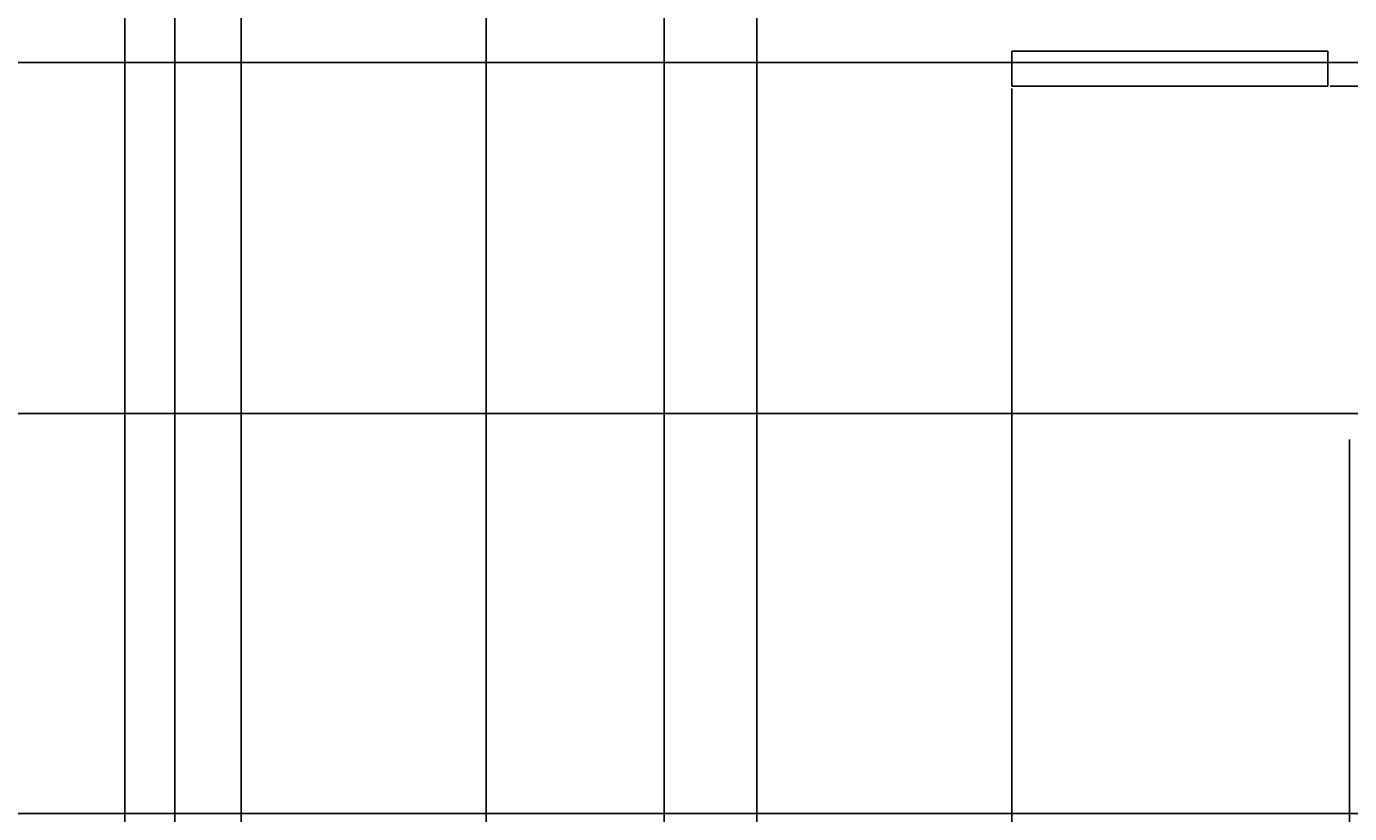
# Model space of a CAD drawing. Units: inches. Extents: x 2812 to 3051, y 1398 to 1659.
# Tile 30 of 65: x 2966 to 3004, y 1416 to 1438. Entities that reach past the tile are written whole.
import ezdxf

# ---------------------------------------------------------------- set-up
doc = ezdxf.new("R2010")
doc.units = ezdxf.units.IN
doc.layers.add('A-ANNO-DIMS', color=2, linetype='Continuous', lineweight=18)
doc.layers.add('S-STEP', color=3, linetype='Continuous', lineweight=25)
doc.styles.get("Standard").update_dxf_attribs({"font": 'arial.ttf'})
doc.dimstyles.get("Standard").update_dxf_attribs({"dimtxt": 0.18, "dimasz": 0.18, "dimexe": 0.18, "dimexo": 0.0625, "dimgap": 0.09, "dimtad": 0, "dimtih": 1, "dimtoh": 1, "dimdec": 4, "dimzin": 0, "dimdsep": 46, "dimtxsty": 'Standard', "dimcen": 0.09, "dimadec": 0, "dimazin": 0, "dimtfac": 1, "dimtdec": 4, "dimtofl": 0, "dimtmove": 0, "dimatfit": 3, "dimfxl": 1, "dimtolj": 1, "dimtzin": 0, "dimarcsym": 0})

# ---------------------------------------------------------------- blocks, each defined once
blk = doc.blocks.new('STEP-IRON-2')
for p, q in [((9, 1), (0, 1)), ((0, 1), (0, 0)), ((9, 0), (9, 1)), ((0, 0), (3.641, 0)), ((0, 0), (9, 0)), ((0, 0), (5.792, 0))]:
    blk.add_line(p, q)
blk = doc.blocks.new('*D31')
at = {"layer": 'A-ANNO-DIMS', "color": 0, "lineweight": -2, "transparency": 16777216}
for p, q in [((2972.272, 1594.192), (2972.272, 1397.505)), ((2961.385, 1559.757), (2961.385, 1397.505)), ((2961.565, 1397.685), (2966.373, 1397.685)), ((2972.092, 1397.685), (2967.283, 1397.685))]:
    blk.add_line(p, q, dxfattribs=at)
at = {"layer": 'A-ANNO-DIMS', "color": 0, "transparency": 16777216}
for points in [[(2961.565, 1397.715), (2961.565, 1397.655), (2961.385, 1397.685)], [(2972.092, 1397.715), (2972.092, 1397.655), (2972.272, 1397.685)]]:
    blk.add_solid(points, dxfattribs=at)
at = {"layer": 'Defpoints', "color": 0, "transparency": 16777216}
for p in [(2972.272, 1594.254), (2961.385, 1559.82), (2972.272, 1397.685)]:
    blk.add_point(p, dxfattribs=at)
at = {"layer": 'A-ANNO-DIMS', "color": 0, "transparency": 16777216, "insert": (2966.828, 1397.685), "char_height": 0.18, "attachment_point": 5}
blk.add_mtext('\\A1;10.887', dxfattribs=at)
blk = doc.blocks.new('*D32')
at = {"layer": 'A-ANNO-DIMS', "color": 0, "lineweight": -2, "transparency": 16777216}
for p, q in [((2984.316, 1598.757), (2984.316, 1397.505)), ((2972.272, 1594.192), (2972.272, 1397.505)), ((2972.452, 1397.685), (2977.839, 1397.685)), ((2984.136, 1397.685), (2978.748, 1397.685))]:
    blk.add_line(p, q, dxfattribs=at)
at = {"layer": 'A-ANNO-DIMS', "color": 0, "transparency": 16777216}
for points in [[(2972.452, 1397.715), (2972.452, 1397.655), (2972.272, 1397.685)], [(2984.136, 1397.715), (2984.136, 1397.655), (2984.316, 1397.685)]]:
    blk.add_solid(points, dxfattribs=at)
at = {"layer": 'Defpoints', "color": 0, "transparency": 16777216}
for p in [(2984.316, 1598.82), (2972.272, 1594.254), (2984.316, 1397.685)]:
    blk.add_point(p, dxfattribs=at)
at = {"layer": 'A-ANNO-DIMS', "color": 0, "transparency": 16777216, "insert": (2978.294, 1397.685), "char_height": 0.18, "attachment_point": 5}
blk.add_mtext('\\A1;12.044', dxfattribs=at)
blk = doc.blocks.new('*D46')
at = {"layer": 'A-ANNO-DIMS', "color": 0, "lineweight": -2, "transparency": 16777216}
for p, q in [((2941.385, 1487.973), (2941.385, 1397.505)), ((2970.385, 1487.973), (2970.385, 1397.505)), ((2941.565, 1397.685), (2955.664, 1397.685)), ((2970.205, 1397.685), (2956.106, 1397.685))]:
    blk.add_line(p, q, dxfattribs=at)
at = {"layer": 'A-ANNO-DIMS', "color": 0, "transparency": 16777216}
for points in [[(2941.565, 1397.715), (2941.565, 1397.655), (2941.385, 1397.685)], [(2970.205, 1397.715), (2970.205, 1397.655), (2970.385, 1397.685)]]:
    blk.add_solid(points, dxfattribs=at)
at = {"layer": 'Defpoints', "color": 0, "transparency": 16777216}
for p in [(2941.385, 1488.035), (2970.385, 1488.035), (2970.385, 1397.685)]:
    blk.add_point(p, dxfattribs=at)
at = {"layer": 'A-ANNO-DIMS', "color": 0, "transparency": 16777216, "insert": (2955.885, 1397.685), "char_height": 0.18, "attachment_point": 5}
blk.add_mtext('\\A1;29', dxfattribs=at)
blk = doc.blocks.new('*D47')
at = {"layer": 'A-ANNO-DIMS', "color": 0, "lineweight": -2, "transparency": 16777216}
for p, q in [((2970.385, 1487.973), (2970.385, 1397.505)), ((3006.385, 1487.973), (3006.385, 1397.505)), ((2970.565, 1397.685), (2988.166, 1397.685)), ((3006.205, 1397.685), (2988.604, 1397.685))]:
    blk.add_line(p, q, dxfattribs=at)
at = {"layer": 'A-ANNO-DIMS', "color": 0, "transparency": 16777216}
for points in [[(2970.565, 1397.715), (2970.565, 1397.655), (2970.385, 1397.685)], [(3006.205, 1397.715), (3006.205, 1397.655), (3006.385, 1397.685)]]:
    blk.add_solid(points, dxfattribs=at)
at = {"layer": 'Defpoints', "color": 0, "transparency": 16777216}
for p in [(2970.385, 1488.035), (3006.385, 1488.035), (3006.385, 1397.685)]:
    blk.add_point(p, dxfattribs=at)
at = {"layer": 'A-ANNO-DIMS', "color": 0, "transparency": 16777216, "insert": (2988.385, 1397.685), "char_height": 0.18, "attachment_point": 5}
blk.add_mtext('\\A1;36', dxfattribs=at)
blk = doc.blocks.new('*D64')
at = {"layer": 'A-ANNO-DIMS', "color": 0, "lineweight": -2, "transparency": 16777216}
for p, q in [((2929.438, 1427.426), (3051.178, 1427.426)), ((3050.998, 1427.246), (3050.998, 1421.913)), ((3050.998, 1416.215), (3050.998, 1421.549)), ((2952.447, 1416.035), (3051.178, 1416.035))]:
    blk.add_line(p, q, dxfattribs=at)
at = {"layer": 'A-ANNO-DIMS', "color": 0, "transparency": 16777216}
for points in [[(3050.968, 1427.246), (3051.028, 1427.246), (3050.998, 1427.426)], [(3050.968, 1416.215), (3051.028, 1416.215), (3050.998, 1416.035)]]:
    blk.add_solid(points, dxfattribs=at)
at = {"layer": 'Defpoints', "color": 0, "transparency": 16777216}
for p in [(2929.375, 1427.426), (3050.998, 1427.426), (2952.385, 1416.035)]:
    blk.add_point(p, dxfattribs=at)
at = {"layer": 'A-ANNO-DIMS', "color": 0, "transparency": 16777216, "insert": (3050.998, 1421.731), "char_height": 0.18, "attachment_point": 5}
blk.add_mtext('\\A1;11.39', dxfattribs=at)
blk = doc.blocks.new('*D65')
at = {"layer": 'A-ANNO-DIMS', "color": 0, "lineweight": -2, "transparency": 16777216}
for p, q in [((2920.62, 1437.426), (3051.178, 1437.426)), ((3050.998, 1437.246), (3050.998, 1432.608)), ((3050.998, 1427.606), (3050.998, 1432.245)), ((2929.438, 1427.426), (3051.178, 1427.426))]:
    blk.add_line(p, q, dxfattribs=at)
at = {"layer": 'A-ANNO-DIMS', "color": 0, "transparency": 16777216}
for points in [[(3050.968, 1437.246), (3051.028, 1437.246), (3050.998, 1437.426)], [(3050.968, 1427.606), (3051.028, 1427.606), (3050.998, 1427.426)]]:
    blk.add_solid(points, dxfattribs=at)
at = {"layer": 'Defpoints', "color": 0, "transparency": 16777216}
for p in [(2920.558, 1437.426), (3050.998, 1437.426), (2929.375, 1427.426)]:
    blk.add_point(p, dxfattribs=at)
at = {"layer": 'A-ANNO-DIMS', "color": 0, "transparency": 16777216, "insert": (3050.998, 1432.426), "char_height": 0.18, "attachment_point": 5}
blk.add_mtext('\\A1;10', dxfattribs=at)
blk = doc.blocks.new('*D66')
at = {"layer": 'A-ANNO-DIMS', "color": 0, "lineweight": -2, "transparency": 16777216}
for p, q in [((2914.018, 1447.426), (3051.178, 1447.426)), ((3050.998, 1447.246), (3050.998, 1442.608)), ((3050.998, 1437.606), (3050.998, 1442.245)), ((2920.62, 1437.426), (3051.178, 1437.426))]:
    blk.add_line(p, q, dxfattribs=at)
at = {"layer": 'A-ANNO-DIMS', "color": 0, "transparency": 16777216}
for points in [[(3050.968, 1447.246), (3051.028, 1447.246), (3050.998, 1447.426)], [(3050.968, 1437.606), (3051.028, 1437.606), (3050.998, 1437.426)]]:
    blk.add_solid(points, dxfattribs=at)
at = {"layer": 'Defpoints', "color": 0, "transparency": 16777216}
for p in [(2913.955, 1447.426), (3050.998, 1447.426), (2920.558, 1437.426)]:
    blk.add_point(p, dxfattribs=at)
at = {"layer": 'A-ANNO-DIMS', "color": 0, "transparency": 16777216, "insert": (3050.998, 1442.426), "char_height": 0.18, "attachment_point": 5}
blk.add_mtext('\\A1;10', dxfattribs=at)
blk = doc.blocks.new('*D71')
at = {"layer": 'A-ANNO-DIMS', "color": 0, "lineweight": -2, "transparency": 16777216}
for p, q in [((2968.956, 1466.685), (2968.956, 1397.505)), ((2979.248, 1456.685), (2979.248, 1397.505)), ((2969.136, 1397.685), (2973.648, 1397.685)), ((2979.068, 1397.685), (2974.556, 1397.685))]:
    blk.add_line(p, q, dxfattribs=at)
at = {"layer": 'A-ANNO-DIMS', "color": 0, "transparency": 16777216}
for points in [[(2969.136, 1397.715), (2969.136, 1397.655), (2968.956, 1397.685)], [(2979.068, 1397.715), (2979.068, 1397.655), (2979.248, 1397.685)]]:
    blk.add_solid(points, dxfattribs=at)
at = {"layer": 'Defpoints', "color": 0, "transparency": 16777216}
for p in [(2968.956, 1466.747), (2979.248, 1456.747), (2979.248, 1397.685)]:
    blk.add_point(p, dxfattribs=at)
at = {"layer": 'A-ANNO-DIMS', "color": 0, "transparency": 16777216, "insert": (2974.102, 1397.685), "char_height": 0.18, "attachment_point": 5}
blk.add_mtext('\\A1;10.292', dxfattribs=at)
blk = doc.blocks.new('*D72')
at = {"layer": 'A-ANNO-DIMS', "color": 0, "lineweight": -2, "transparency": 16777216}
for p, q in [((2979.248, 1456.685), (2979.248, 1397.505)), ((2986.956, 1446.685), (2986.956, 1397.505)), ((2979.428, 1397.685), (2982.709, 1397.685)), ((2986.776, 1397.685), (2983.495, 1397.685))]:
    blk.add_line(p, q, dxfattribs=at)
at = {"layer": 'A-ANNO-DIMS', "color": 0, "transparency": 16777216}
for points in [[(2979.428, 1397.715), (2979.428, 1397.655), (2979.248, 1397.685)], [(2986.776, 1397.715), (2986.776, 1397.655), (2986.956, 1397.685)]]:
    blk.add_solid(points, dxfattribs=at)
at = {"layer": 'Defpoints', "color": 0, "transparency": 16777216}
for p in [(2979.248, 1456.747), (2986.956, 1446.747), (2986.956, 1397.685)]:
    blk.add_point(p, dxfattribs=at)
at = {"layer": 'A-ANNO-DIMS', "color": 0, "transparency": 16777216, "insert": (2983.102, 1397.685), "char_height": 0.18, "attachment_point": 5}
blk.add_mtext('\\A1;7.708', dxfattribs=at)
blk = doc.blocks.new('*D73')
at = {"layer": 'A-ANNO-DIMS', "color": 0, "lineweight": -2, "transparency": 16777216}
for p, q in [((2986.956, 1446.685), (2986.956, 1397.505)), ((2994.221, 1436.685), (2994.221, 1397.505)), ((2987.136, 1397.685), (2990.195, 1397.685)), ((2994.041, 1397.685), (2990.982, 1397.685))]:
    blk.add_line(p, q, dxfattribs=at)
at = {"layer": 'A-ANNO-DIMS', "color": 0, "transparency": 16777216}
for points in [[(2987.136, 1397.715), (2987.136, 1397.655), (2986.956, 1397.685)], [(2994.041, 1397.715), (2994.041, 1397.655), (2994.221, 1397.685)]]:
    blk.add_solid(points, dxfattribs=at)
at = {"layer": 'Defpoints', "color": 0, "transparency": 16777216}
for p in [(2986.956, 1446.747), (2994.221, 1436.747), (2994.221, 1397.685)]:
    blk.add_point(p, dxfattribs=at)
at = {"layer": 'A-ANNO-DIMS', "color": 0, "transparency": 16777216, "insert": (2990.589, 1397.685), "char_height": 0.18, "attachment_point": 5}
blk.add_mtext('\\A1;7.265', dxfattribs=at)
blk = doc.blocks.new('*D74')
at = {"layer": 'A-ANNO-DIMS', "color": 0, "lineweight": -2, "transparency": 16777216}
for p, q in [((2994.221, 1436.685), (2994.221, 1397.505)), ((3003.837, 1426.685), (3003.837, 1397.505)), ((2994.401, 1397.685), (2998.635, 1397.685)), ((3003.657, 1397.685), (2999.423, 1397.685))]:
    blk.add_line(p, q, dxfattribs=at)
at = {"layer": 'A-ANNO-DIMS', "color": 0, "transparency": 16777216}
for points in [[(2994.401, 1397.715), (2994.401, 1397.655), (2994.221, 1397.685)], [(3003.657, 1397.715), (3003.657, 1397.655), (3003.837, 1397.685)]]:
    blk.add_solid(points, dxfattribs=at)
at = {"layer": 'Defpoints', "color": 0, "transparency": 16777216}
for p in [(2994.221, 1436.747), (3003.837, 1426.747), (3003.837, 1397.685)]:
    blk.add_point(p, dxfattribs=at)
at = {"layer": 'A-ANNO-DIMS', "color": 0, "transparency": 16777216, "insert": (2999.029, 1397.685), "char_height": 0.18, "attachment_point": 5}
blk.add_mtext('\\A1;9.615', dxfattribs=at)
blk = doc.blocks.new('*D79')
at = {"layer": 'A-ANNO-DIMS', "color": 0, "lineweight": -2, "transparency": 16777216}
for p, q in [((3003.284, 1436.747), (3051.178, 1436.747)), ((3050.998, 1436.567), (3050.998, 1431.929)), ((3050.998, 1426.927), (3050.998, 1431.565)), ((3012.899, 1426.747), (3051.178, 1426.747))]:
    blk.add_line(p, q, dxfattribs=at)
at = {"layer": 'A-ANNO-DIMS', "color": 0, "transparency": 16777216}
for points in [[(3050.968, 1436.567), (3051.028, 1436.567), (3050.998, 1436.747)], [(3050.968, 1426.927), (3051.028, 1426.927), (3050.998, 1426.747)]]:
    blk.add_solid(points, dxfattribs=at)
at = {"layer": 'Defpoints', "color": 0, "transparency": 16777216}
for p in [(3003.221, 1436.747), (3050.998, 1436.747), (3012.837, 1426.747)]:
    blk.add_point(p, dxfattribs=at)
at = {"layer": 'A-ANNO-DIMS', "color": 0, "transparency": 16777216, "insert": (3050.998, 1431.747), "char_height": 0.18, "attachment_point": 5}
blk.add_mtext('\\A1;10', dxfattribs=at)
blk = doc.blocks.new('*D80')
at = {"layer": 'A-ANNO-DIMS', "color": 0, "lineweight": -2, "transparency": 16777216}
for p, q in [((2996.018, 1446.747), (3051.178, 1446.747)), ((3050.998, 1446.567), (3050.998, 1441.929)), ((3050.998, 1436.927), (3050.998, 1441.565)), ((3003.284, 1436.747), (3051.178, 1436.747))]:
    blk.add_line(p, q, dxfattribs=at)
at = {"layer": 'A-ANNO-DIMS', "color": 0, "transparency": 16777216}
for points in [[(3050.968, 1446.567), (3051.028, 1446.567), (3050.998, 1446.747)], [(3050.968, 1436.927), (3051.028, 1436.927), (3050.998, 1436.747)]]:
    blk.add_solid(points, dxfattribs=at)
at = {"layer": 'Defpoints', "color": 0, "transparency": 16777216}
for p in [(2995.956, 1446.747), (3050.998, 1446.747), (3003.221, 1436.747)]:
    blk.add_point(p, dxfattribs=at)
at = {"layer": 'A-ANNO-DIMS', "color": 0, "transparency": 16777216, "insert": (3050.998, 1441.747), "char_height": 0.18, "attachment_point": 5}
blk.add_mtext('\\A1;10', dxfattribs=at)

msp = doc.modelspace()

# ---------------------------------------------------------------- block references
at = {"layer": 'S-STEP'}
msp.add_blockref('STEP-IRON-2', (2994.221, 1436.747), dxfattribs=at)

# ---------------------------------------------------------------- dimensions: what is measured, and where the dimension line sits
at = {"layer": 'A-ANNO-DIMS'}
for base, p1, p2, override, picture, middle in [((2984.3156, 1397.6854), (2972.2716, 1594.2541), (2984.3156, 1598.82), {"dimdec": 3, "dimlfac": 1, "dimrnd": 0, "dimzin": 0, "dimdsep": 46, "dimlunit": 2}, '*D32', (2978.2936, 1397.6854)), ((2972.2716, 1397.6854), (2961.3849, 1559.82), (2972.2716, 1594.2541), {"dimdec": 3, "dimlfac": 1, "dimrnd": 0, "dimzin": 0, "dimdsep": 46, "dimlunit": 2}, '*D31', (2966.8282, 1397.6854)), ((2970.3849, 1397.6854), (2941.3849, 1488.0354), (2970.3849, 1488.0354), {"dimdec": 0, "dimlfac": 1, "dimrnd": 0, "dimzin": 0, "dimdsep": 46, "dimlunit": 2}, '*D46', (2955.8849, 1397.6854)), ((3006.3849, 1397.6854), (2970.3849, 1488.0354), (3006.3849, 1488.0354), {"dimdec": 0, "dimlfac": 1, "dimrnd": 0, "dimzin": 0, "dimdsep": 46, "dimlunit": 2}, '*D47', (2988.3849, 1397.6854)), ((2979.2478, 1397.6854), (2968.9558, 1466.7474), (2979.2478, 1456.7474), {"dimdec": 3, "dimlfac": 1, "dimrnd": 0, "dimzin": 0, "dimdsep": 46, "dimlunit": 2}, '*D71', (2974.1018, 1397.6854)), ((2986.9558, 1397.6854), (2979.2478, 1456.7474), (2986.9558, 1446.7474), {"dimdec": 3, "dimlfac": 1, "dimrnd": 0, "dimzin": 0, "dimdsep": 46, "dimlunit": 2}, '*D72', (2983.1018, 1397.6854)), ((2994.22128, 1397.6854), (2986.95585, 1446.74738), (2994.22128, 1436.74738), {"dimdec": 3, "dimlfac": 1, "dimrnd": 0, "dimzin": 0, "dimdsep": 46, "dimlunit": 2}, '*D73', (2990.58856, 1397.6854)), ((3003.83676, 1397.6854), (2994.22128, 1436.74738), (3003.83676, 1426.74738), {"dimdec": 3, "dimlfac": 1, "dimrnd": 0, "dimzin": 0, "dimdsep": 46, "dimlunit": 2}, '*D74', (2999.02902, 1397.6854))]:
    dim = msp.add_linear_dim(base=base, p1=p1, p2=p2, dimstyle='Standard', override=override, dxfattribs=at)
    dim.commit()
    dim.dimension.update_dxf_attribs({"geometry": picture, "text_midpoint": middle})
for base, p1, p2, override, picture, middle in [((3050.998, 1447.4265), (2920.5577, 1437.4265), (2913.9551, 1447.4265), {"dimdec": 0, "dimlfac": 1, "dimrnd": 0, "dimzin": 0, "dimdsep": 46, "dimlunit": 2}, '*D66', (3050.998, 1442.4265)), ((3050.998, 1446.7474), (3003.2213, 1436.7474), (2995.9558, 1446.7474), {"dimdec": 0, "dimlfac": 1, "dimrnd": 0, "dimzin": 0, "dimdsep": 46, "dimlunit": 2}, '*D80', (3050.998, 1441.7474)), ((3050.998, 1437.4265), (2929.3751, 1427.4265), (2920.5577, 1437.4265), {"dimdec": 0, "dimlfac": 1, "dimrnd": 0, "dimzin": 0, "dimdsep": 46, "dimlunit": 2}, '*D65', (3050.998, 1432.4265)), ((3050.998, 1436.7474), (3012.8368, 1426.7474), (3003.2213, 1436.7474), {"dimdec": 0, "dimlfac": 1, "dimrnd": 0, "dimzin": 0, "dimdsep": 46, "dimlunit": 2}, '*D79', (3050.998, 1431.7474)), ((3050.998, 1427.4265), (2952.3849, 1416.0354), (2929.3751, 1427.4265), {"dimdec": 2, "dimlfac": 1, "dimrnd": 0, "dimzin": 0, "dimdsep": 46, "dimlunit": 2}, '*D64', (3050.998, 1421.7309))]:
    dim = msp.add_linear_dim(base=base, p1=p1, p2=p2, angle=90, dimstyle='Standard', override=override, dxfattribs=at)
    dim.commit()
    dim.dimension.update_dxf_attribs({"geometry": picture, "text_midpoint": middle})

doc.saveas('drawing.dxf')
